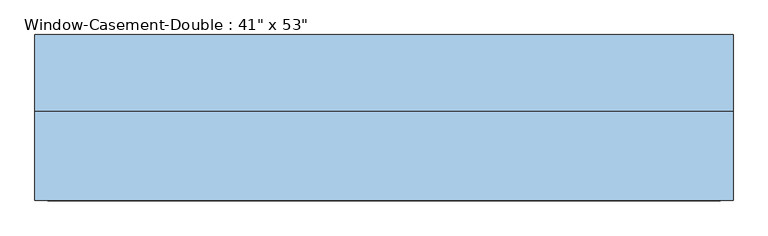
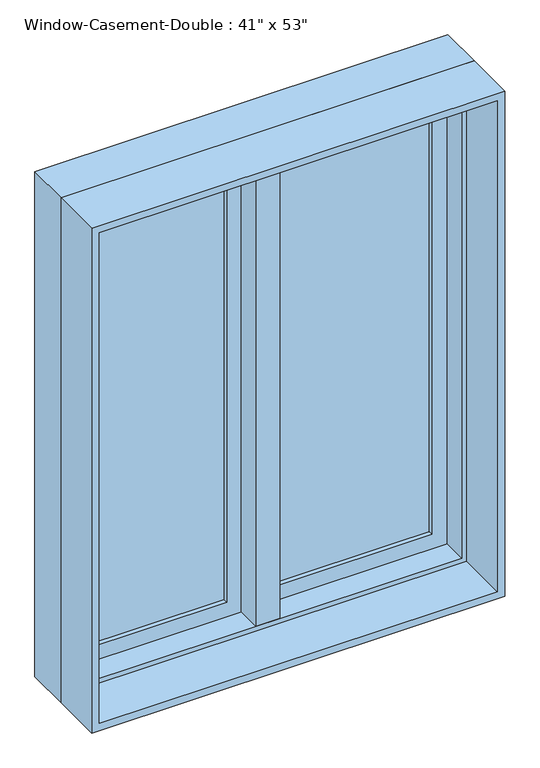
"""IFC4 building model written with IfcOpenShell, lengths in millimetres: window geometry."""

from ifc_helpers import new_model, si_unit, frame, origin, place, context, project, spatial, polyline, outline, extrude, faceted_brep, source, transform, mapped, element, save


def window_c95ebb39(model_context):
    return source(origin(), model_context, "Body", "SolidModel", [
        faceted_brep([(9.525, 133.35, 2247.9), (-9.525, 133.35, 2247.9), (-9.525, 82.55, 2247.9), (9.525, 82.55, 2247.9), (9.525, 133.35, 927.1), (9.525, 82.55, 927.1), (-9.525, 82.55, 927.1), (-9.525, 133.35, 927.1), (-9.525, 82.55, 946.15), (-9.525, 82.55, 2228.85), (-30.1625, 82.55, 946.15), (-30.1625, 82.55, 2228.85), (-30.1625, 19.05, 946.15), (-30.1625, 19.05, 2228.85), (30.1625, 19.05, 946.15), (30.1625, 19.05, 2228.85), (30.1625, 82.55, 946.15), (30.1625, 82.55, 2228.85), (9.525, 82.55, 946.15), (9.525, 82.55, 2228.85)], [[[0, 1, 2, 3]], [[4, 5, 6, 7]], [[1, 0, 4, 7]], [[2, 1, 7, 6, 8, 9]], [[9, 8, 10, 11]], [[11, 10, 12, 13]], [[13, 12, 14, 15]], [[15, 14, 16, 17]], [[17, 16, 18, 19]], [[0, 3, 19, 18, 5, 4]], [[18, 8, 6, 5]], [[9, 19, 3, 2]], [[8, 18, 16, 14, 12, 10]], [[19, 9, 11, 13, 15, 17]]]),
        extrude(outline(polyline([(-66.675, 114.3), (-66.675, 107.95), (-450.85, 107.95), (-450.85, 114.3), (-66.675, 114.3)])), frame((0.0, 0.0, 984.25), z_axis=(0.0, 0.0, 1.0), x_axis=(1.0, 0.0, 0.0)), (0.0, 0.0, 1.0), 1206.5),
        extrude(outline(polyline([(-450.85, 95.25), (-450.85, 101.6), (-66.675, 101.6), (-66.675, 95.25), (-450.85, 95.25)])), frame((0.0, 0.0, 984.25), z_axis=(0.0, 0.0, 1.0), x_axis=(1.0, 0.0, 0.0)), (0.0, 0.0, 1.0), 1206.5),
        extrude(outline(polyline([(450.85, 114.3), (450.85, 107.95), (66.675, 107.95), (66.675, 114.3), (450.85, 114.3)])), frame((0.0, 0.0, 984.25), z_axis=(0.0, 0.0, 1.0), x_axis=(1.0, 0.0, 0.0)), (0.0, 0.0, 1.0), 1206.5),
        extrude(outline(polyline([(66.675, 95.25), (66.675, 101.6), (450.85, 101.6), (450.85, 95.25), (66.675, 95.25)])), frame((0.0, 0.0, 984.25), z_axis=(0.0, 0.0, 1.0), x_axis=(1.0, 0.0, 0.0)), (0.0, 0.0, 1.0), 1206.5),
        extrude(outline(polyline([(2247.9, -508.0), (927.1, -508.0), (927.1, -9.525), (2247.9, -9.525), (2247.9, -508.0)]), holes=[polyline([(2190.75, -66.675), (984.25, -66.675), (984.25, -450.85), (2190.75, -450.85), (2190.75, -66.675)])]), frame((0.0, 82.55, 0.0), z_axis=(0.0, 1.0, 0.0), x_axis=(0.0, 0.0, 1.0)), (0.0, 0.0, 1.0), 44.45),
        extrude(outline(polyline([(927.1, 508.0), (2247.9, 508.0), (2247.9, 9.525), (927.1, 9.525), (927.1, 508.0)]), holes=[polyline([(984.25, 66.675), (2190.75, 66.675), (2190.75, 450.85), (984.25, 450.85), (984.25, 66.675)])]), frame((0.0, 82.55, 0.0), z_axis=(0.0, 1.0, 0.0), x_axis=(0.0, 0.0, 1.0)), (0.0, 0.0, 1.0), 44.45),
        extrude(outline(polyline([(2260.6, -520.7), (914.4, -520.7), (914.4, 520.7), (2260.6, 520.7), (2260.6, -520.7)]), holes=[polyline([(2241.55, 501.65), (933.45, 501.65), (933.45, -501.65), (2241.55, -501.65), (2241.55, 501.65)])]), frame((0.0, -114.3, 0.0), z_axis=(0.0, 1.0, 0.0), x_axis=(0.0, 0.0, 1.0)), (0.0, 0.0, 1.0), 133.35),
        faceted_brep([(488.95, 82.55, 2228.85), (488.95, 19.05, 2228.85), (-488.95, 19.05, 2228.85), (-488.95, 82.55, 2228.85), (508.0, 133.35, 2247.9), (508.0, 82.55, 2247.9), (-508.0, 82.55, 2247.9), (-508.0, 133.35, 2247.9), (520.7, 19.05, 2260.6), (520.7, 133.35, 2260.6), (-520.7, 133.35, 2260.6), (-520.7, 19.05, 2260.6), (-488.95, 19.05, 946.15), (-488.95, 82.55, 946.15), (-508.0, 82.55, 927.1), (-508.0, 133.35, 927.1), (-520.7, 133.35, 914.4), (-520.7, 19.05, 914.4), (488.95, 19.05, 946.15), (488.95, 82.55, 946.15), (508.0, 82.55, 927.1), (508.0, 133.35, 927.1), (520.7, 133.35, 914.4), (520.7, 19.05, 914.4)], [[[0, 1, 2, 3]], [[4, 5, 6, 7]], [[8, 9, 10, 11]], [[3, 2, 12, 13]], [[7, 6, 14, 15]], [[11, 10, 16, 17]], [[13, 12, 18, 19]], [[15, 14, 20, 21]], [[17, 16, 22, 23]], [[11, 17, 23, 8], [1, 18, 12, 2]], [[19, 18, 1, 0]], [[5, 20, 14, 6], [3, 13, 19, 0]], [[21, 20, 5, 4]], [[23, 22, 9, 8]], [[9, 22, 16, 10], [7, 15, 21, 4]]]),
    ])


if __name__ == "__main__":
    model = new_model("IFC4")
    model_context = context("Model", 3, world=origin())
    ifc_project = project(units=[si_unit("LENGTHUNIT", "METRE", prefix="MILLI")], contexts=[model_context])
    site = spatial("IfcSite", under=ifc_project)
    building = spatial("IfcBuilding", under=site)
    placement = place(None, origin())
    window_shape = window_c95ebb39(model_context)
    element("IfcWindow", 1, ObjectType="Window-Casement-Double : 41\" x 53\"", at=placement, inside=building, context=model_context, shape_type="MappedRepresentation", body=[
        mapped(window_shape, transform((0.0, 0.0, 0.0), x_axis=(1.0, 0.0, 0.0), y_axis=(0.0, 1.0, 0.0), z_axis=(0.0, 0.0, 1.0))),
    ])
    save(model, "model.ifc")

# Revit data of these elements
# Type "Window-Casement-Double : 41\" x 53\""
#   Type Mark = "15"
#   Fire Rating = "0.5h"
#   Assembly Code = "B2020100"
#   Analytic Construction = "Double glazing - domestic"
#   Frame Extension [instance default] = 0' - 0 1/4"
#   Window Inset [instance default] = 0' - 0"
#   Wall Thickness [instance default] = 0' - 6"
#   Interior Wall Closure [instance default] = 0' - 2 1/4"
#   Half Width = 1' - 8 1/2"
#   Visual Light Transmittance = 0.81
#   Thermal Resistance (R) = 1.8146 (h·ft²·°F)/BTU
#   Solar Heat Gain Coefficient = 0.76
#   Rough Width = 3' - 5 1/2"
#   Rough Height = 4' - 5 1/2"
#   Height = 4' - 5"
#   Heat Transfer Coefficient (U) = 0.5511 BTU/(h·ft²·°F)
#   Exterior Wall Closure [instance default] = 0' - 1 1/4"
#   Extension Jamb [instance default] = 0' - 2 1/4"
#   Default Sill Height = 3' - 0"
#   Width = 3' - 5"
#   Define Thermal Properties by = 0
#   Muntin Visibility = yes
#   Interior Trim Visibility [instance default] = yes
#   Exterior Trim Visibility [instance default] = yes
#   Extension Jamb Visibility [instance default] = yes
#   Interior Trim Material = Wood - Stained
#   Muntin Pattern = Muntin Pattern_2x2 : Muntin Pattern_2x2
#   Interior Trim = Trim-Window-Interior-Flat : Picture Frame
#   Interior Frame Material = Wood - Stained
#   Glass Panel Material = Glass
#   Exterior Trim Material = Clad - White
#   Exterior Trim = Trim-Window-Exterior-Flat : with Sill
#   Exterior Frame Material = Clad - White
#   Wall Closure = (empty or 0)
# Element 1 (IfcWindow, "Window-Casement-Double : 41\" x 53\"")
#   Wall Thickness = 0' - 9"
#   Extension Jamb = 0' - 5 1/4"
#   Materials on its faces: "Wood - Stained", "Glass", "Clad - White"
# Materials
#   "Wood - Stained": class "Wood", colour RGB 224 178 126, transparency 0, Cost = 0
#   "Glass": class "Glass", colour RGB 0 128 192, transparency 0.75, Description = "Soda Lime Glass", Cost = 0
#   "Clad - White": class "Wood", colour RGB 30 30 30, transparency 0, Cost = 0
